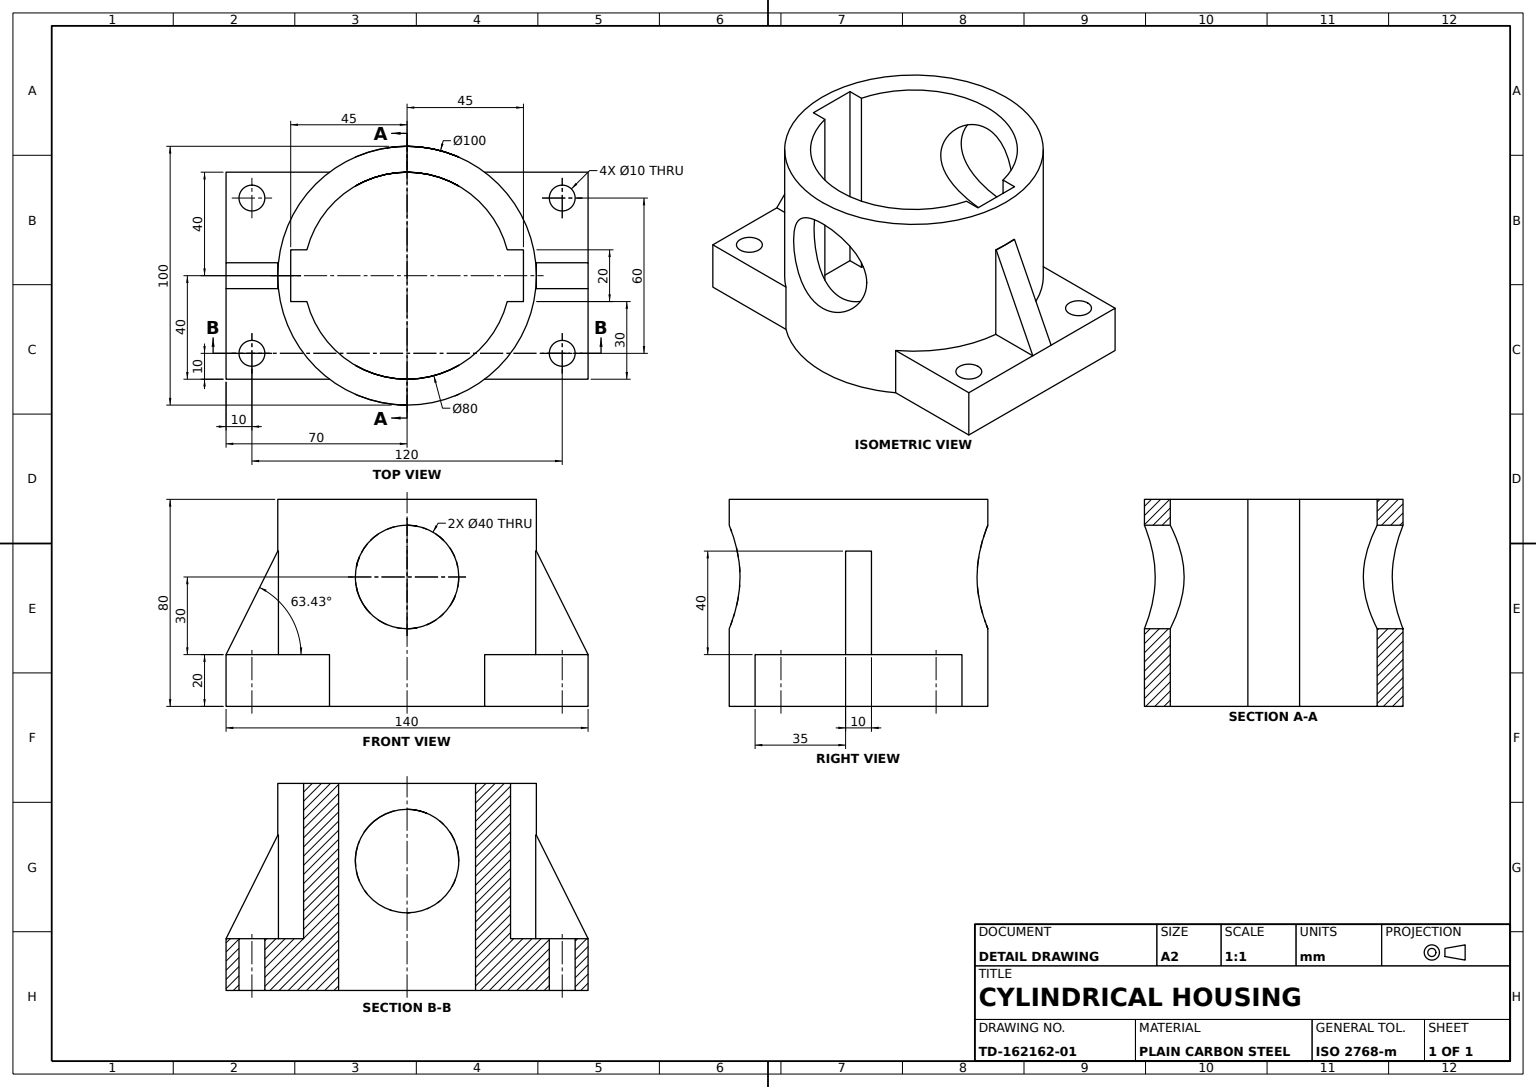
SolidWorks part; units mm, degrees
material "Plain Carbon Steel"
ref_plane "Front Plane" through (0, 0, 0) normal (0, 0, 1) x (1, 0, 0)
ref_plane "Top Plane" through (0, 0, 0) normal (0, 1, 0) x (1, 0, 0)
ref_plane "Right Plane" through (0, 0, 0) normal (1, 0, 0) x (0, 0, -1)
sketch "Housing Profile Sketch" plane through (0, 0, 0) normal (0, 1, 0) x (1, 0, 0)
  line L0 (-38.7298, 10) -> (-45, 10)
  line L1 (-45, 10) -> (-45, -10)
  line L2 (-45, -10) -> (-38.7298, -10)
  line L3 (0, 0) -> (0, -20.1306) construction
  line L4 (45, -10) -> (38.7298, -10)
  line L5 (45, 10) -> (45, -10)
  line L6 (38.7298, 10) -> (45, 10)
  circle A0 centre (0, 0) radius 50
  arc A1 (-38.7298, -10) -> (38.7298, -10) centre (0, 0) ccw
  arc A2 (38.7298, 10) -> (-38.7298, 10) centre (0, 0) ccw
  point P6 (-45, 0)
  point P13 (45, 0)
  dimension "D1" = 100
  dimension "D2" = 80
  dimension "D3" = 45
  dimension "D4" = 20
extrude "Housing Body" add sketch "Housing Profile Sketch" along normal blind 80
sketch "Base Flange Sketch" plane through (0, 0, 0) normal (0, -1, 0) x (1, 0, 0)
  line L0 (30, 40) -> (70, 40)
  line L1 (-70, -40) -> (-30, -40)
  line L2 (-70, -40) -> (-70, 40)
  line L3 (-70, 40) -> (-30, 40)
  line L4 (70, -40) -> (70, 40)
  line L5 (-70, -40) -> (70, 40) construction
  line L6 (-70, 40) -> (70, -40) construction
  line L7 (30, -40) -> (70, -40)
  circle A0 centre (0, 0) radius 50 construction
  arc A1 (-30, 40) -> (-30, -40) centre (0, 0) ccw
  arc A2 (30, -40) -> (30, 40) centre (0, 0) ccw
  point P0 (0, 0)
  dimension "D1" = 80
  dimension "D2" = 140
extrude "Base Flange" add sketch "Base Flange Sketch" against normal blind 20
sketch "Support Rib Sketch" plane through (0, 0, 0) normal (0, 0, 1) x (1, 0, 0)
  line L0 (-50, 60) -> (-70.0093, 20)
  line L1 (-50, 80) -> (-50, 20) construction
  line L3 (-30, 20) -> (-70, 20) construction
  line L4 (-50, 20) -> (-70.0093, 20)
  line L5 (-50, 60) -> (-48.1253, 60)
  line L6 (-48.1253, 60) -> (-48.1253, 20)
  line L7 (-48.1253, 20) -> (-50, 20)
  dimension "D1" = 40
  dimension "D2" = 63.424
  dimension "D3" = 1.8747
extrude "Support Rib" add sketch "Support Rib Sketch" along normal mid plane 10
mirror "Support Rib Mirror" about plane through (0, 0, 0) normal (1, 0, 0) of "Support Rib"
sketch "Cross Bore Sketch" plane through (0, 0, 0) normal (0, 0, 1) x (1, 0, 0)
  line L0 (38.7298, 80) -> (-38.7298, 80) construction
  circle A0 centre (0, 50) radius 20
  dimension "D1" = 40
  dimension "D2" = 30
extrude "Cross Bore Ø40" cut sketch "Cross Bore Sketch" against normal through all both and the other way through all
sketch "Mounting Holes Sketch" plane through (0, 20, 0) normal (0, 1, 0) x (1, 0, 0)
  circle A0 centre (-60, 30) radius 5
  circle A1 centre (60, 30) radius 5
  circle A2 centre (60, -30) radius 5
  circle A3 centre (-60, -30) radius 5
  dimension "D1" = 10
  dimension "D2" = 30
  dimension "D3" = 60
  dimension "D6" = 60
  dimension "D7" = 120
  dimension "D4" = 2
  dimension "D5" = 2
extrude "Mounting Holes 4xØ10" cut sketch "Mounting Holes Sketch" against normal up to next
